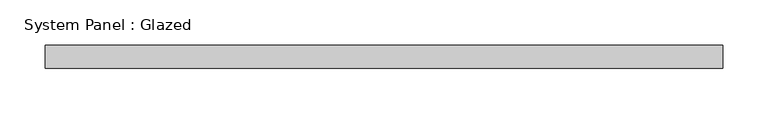
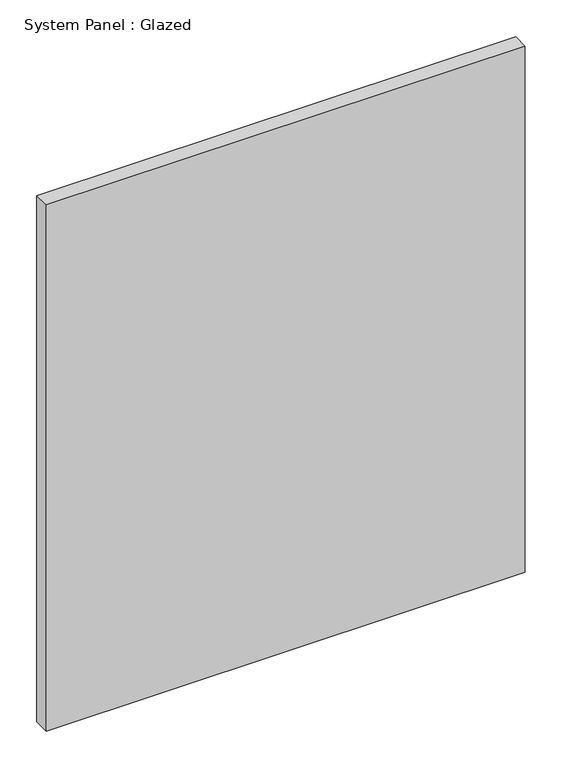
"""IFC4 building model written with IfcOpenShell, lengths in millimetres: plate geometry, System Panel : Glazed."""

from ifc_helpers import new_model, si_unit, origin, origin_with_axes, place, context, project, spatial, polyline, outline, extrude, source, transform, mapped, element, save


def system_panel_glazed_a3e6f34c(model_context):
    return source(origin(), model_context, "Body", "SweptSolid", [
        extrude(outline(polyline([(374.65, 19.05), (-374.65, 19.05), (-374.65, 44.45), (374.65, 44.45), (374.65, 19.05)])), origin_with_axes(), (0.0, 0.0, 1.0), 869.95),
    ])


if __name__ == "__main__":
    model = new_model("IFC4")
    model_context = context("Model", 3, world=origin())
    ifc_project = project(units=[si_unit("LENGTHUNIT", "METRE", prefix="MILLI")], contexts=[model_context])
    site = spatial("IfcSite", under=ifc_project)
    building = spatial("IfcBuilding", under=site)
    placement = place(None, origin())
    system_panel_glazed_shape = system_panel_glazed_a3e6f34c(model_context)
    element("IfcPlate", 1, ObjectType="System Panel : Glazed", at=placement, inside=building, context=model_context, shape_type="MappedRepresentation", body=[
        mapped(system_panel_glazed_shape, transform((0.0, 0.0, 0.0), x_axis=(1.0, 0.0, 0.0), y_axis=(0.0, 1.0, 0.0), z_axis=(0.0, 0.0, 1.0))),
    ])
    save(model, "model.ifc")

# Revit data of these elements
# Type "System Panel : Glazed"
#   Construction Type Id = "GSP4R"
#   Analytic Construction = "1/8 in Pilkington single glazing"
#   Visual Light Transmittance = 0.9
#   Solar Heat Gain Coefficient = 0.86
#   Heat Transfer Coefficient (U) = 1.18115 BTU/(h·ft²·°F)
#   Define Thermal Properties by = 1
# Element 1 (IfcPlate, "System Panel : Glazed")
#   Materials on its faces: "Glass"
# Materials
#   "Glass": class "Glass", colour RGB 0 128 192, transparency 0.75, Description = "Soda Lime Glass", Cost = 0
